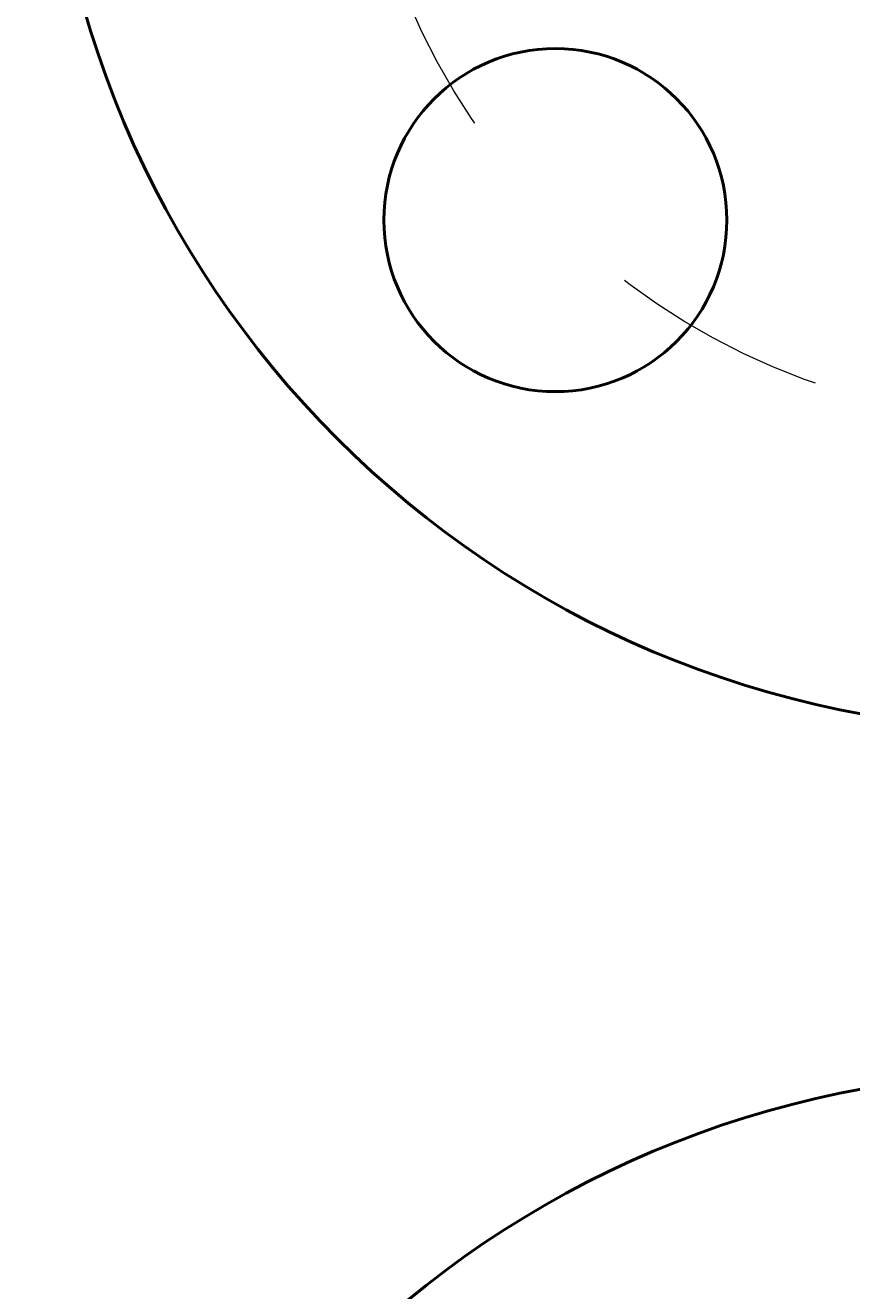
# Model space of a CAD drawing. Units: inches. Extents: x -11 to 126, y -62 to 82.
# Tile 7 of 10: x 30 to 54, y 1 to 38. Entities that reach past the tile are written whole.
import ezdxf

# ---------------------------------------------------------------- set-up
doc = ezdxf.new("R2010")
doc.units = ezdxf.units.IN
doc.header["$MEASUREMENT"] = 0
doc.linetypes.add('CENTER', pattern=[50.8, 31.75, -6.35, 6.35, -6.35])
for name, color, linetype, lineweight in [('M-CNTR', 4, 'CENTER', 18), ('M-DIMS', 2, 'Continuous', 18), ('M-OUTL', 7, 'Continuous', 50)]:
    doc.layers.add(name, color=color, linetype=linetype, lineweight=lineweight)
doc.styles.get("Standard").update_dxf_attribs({"font": 'arial.ttf'})
doc.dimstyles.get("Standard").update_dxf_attribs({"dimtxt": 0.18, "dimasz": 0.18, "dimexe": 0.18, "dimexo": 0.0625, "dimgap": 0.09, "dimtad": 0, "dimtih": 1, "dimtoh": 1, "dimdec": 4, "dimzin": 0, "dimdsep": 46, "dimtxsty": 'Standard', "dimcen": 0.09, "dimadec": 0, "dimazin": 0, "dimtfac": 1, "dimtdec": 4, "dimtofl": 0, "dimtmove": 0, "dimatfit": 3, "dimfxl": 1, "dimtolj": 1, "dimtzin": 0, "dimarcsym": 0})

# ---------------------------------------------------------------- blocks, each defined once
blk = doc.blocks.new('*U1')
blk.add_circle((0, 0), 5)
blk = doc.blocks.new('*U2')
at = {"layer": 'M-OUTL', "color": 0, "linetype": 'ByBlock', "lineweight": -2, "transparency": 16777216, "rotation": 315.0000000000001}
blk.add_blockref('*U1', (45.089, 32.212), dxfattribs=at)
blk = doc.blocks.new('*D5')
at = {"layer": 'Defpoints', "color": 0, "transparency": 16777216}
for p in [(119.232, 12.354), (-0.749, 11.479), (119.232, -57.296)]:
    blk.add_point(p, dxfattribs=at)
at = {"layer": 'M-DIMS', "color": 0, "lineweight": -2, "transparency": 16777216}
for p, q in [((119.232, 12.292), (119.232, -57.476)), ((-0.749, 11.416), (-0.749, -57.476)), ((-0.569, -57.296), (58.786, -57.296)), ((119.052, -57.296), (59.696, -57.296))]:
    blk.add_line(p, q, dxfattribs=at)
at = {"layer": 'M-DIMS', "color": 0, "transparency": 16777216}
for points in [[(-0.569, -57.266), (-0.569, -57.326), (-0.749, -57.296)], [(119.052, -57.266), (119.052, -57.326), (119.232, -57.296)]]:
    blk.add_solid(points, dxfattribs=at)
at = {"layer": 'M-DIMS', "color": 0, "transparency": 16777216, "insert": (59.241, -57.296), "char_height": 0.18, "attachment_point": 5}
blk.add_mtext('\\A1;119.98', dxfattribs=at)
blk = doc.blocks.new('*D6')
at = {"layer": 'Defpoints', "color": 0, "transparency": 16777216}
for p in [(-7.399, 75.354), (59.232, 75.354), (59.232, -50.646)]:
    blk.add_point(p, dxfattribs=at)
at = {"layer": 'M-DIMS', "color": 0, "lineweight": -2, "transparency": 16777216}
for p, q in [((59.169, 75.354), (-7.579, 75.354)), ((-7.399, 75.174), (-7.399, 12.536)), ((-7.399, -50.466), (-7.399, 12.172)), ((59.169, -50.646), (-7.579, -50.646))]:
    blk.add_line(p, q, dxfattribs=at)
at = {"layer": 'M-DIMS', "color": 0, "transparency": 16777216}
for points in [[(-7.429, 75.174), (-7.369, 75.174), (-7.399, 75.354)], [(-7.429, -50.466), (-7.369, -50.466), (-7.399, -50.646)]]:
    blk.add_solid(points, dxfattribs=at)
at = {"layer": 'M-DIMS', "color": 0, "transparency": 16777216, "insert": (-7.399, 12.354), "char_height": 0.18, "attachment_point": 5}
blk.add_mtext('\\A1;126', dxfattribs=at)
blk = doc.blocks.new('*D7')
at = {"layer": 'Defpoints', "color": 0, "transparency": 16777216}
for p in [(59.232, 82.004), (59.232, 46.354), (19.232, 12.354)]:
    blk.add_point(p, dxfattribs=at)
at = {"layer": 'M-DIMS', "color": 0, "lineweight": -2, "transparency": 16777216}
for p, q in [((19.232, 12.417), (19.232, 82.184)), ((19.412, 82.004), (39.009, 82.004)), ((59.052, 82.004), (39.454, 82.004)), ((59.232, 46.417), (59.232, 82.184))]:
    blk.add_line(p, q, dxfattribs=at)
at = {"layer": 'M-DIMS', "color": 0, "transparency": 16777216}
for points in [[(19.412, 82.034), (19.412, 81.974), (19.232, 82.004)], [(59.052, 82.034), (59.052, 81.974), (59.232, 82.004)]]:
    blk.add_solid(points, dxfattribs=at)
at = {"layer": 'M-DIMS', "color": 0, "transparency": 16777216, "insert": (39.232, 82.004), "char_height": 0.18, "attachment_point": 5}
blk.add_mtext('\\A1;40', dxfattribs=at)
blk = doc.blocks.new('*D13')
at = {"layer": 'Defpoints', "color": 0, "transparency": 16777216}
for p in [(73.731, 3.469), (44.732, -46.761)]:
    blk.add_point(p, dxfattribs=at)
at = {"layer": 'M-DIMS', "color": 0, "lineweight": -2, "transparency": 16777216}
for p, q in [((59.142, -21.646), (59.322, -21.646)), ((59.232, -21.736), (59.232, -21.556)), ((36.032, -61.83), (44.642, -46.917)), ((35.852, -61.83), (36.032, -61.83))]:
    blk.add_line(p, q, dxfattribs=at)
at = {"layer": 'M-DIMS', "color": 0, "transparency": 16777216}
blk.add_solid([(44.616, -46.902), (44.668, -46.932), (44.732, -46.761)], dxfattribs=at)
at = {"layer": 'M-DIMS', "color": 0, "transparency": 16777216, "insert": (35.345, -61.83), "char_height": 0.18, "attachment_point": 5}
blk.add_mtext('\\A1;2X ∅58', dxfattribs=at)

msp = doc.modelspace()

# ---------------------------------------------------------------- linework, layer by layer
at = {"layer": 'M-CNTR'}
msp.add_circle((59.232, 46.354), 20, dxfattribs=at)
at = {"layer": 'M-OUTL'}
for centre in [(59.232, 46.354), (59.232, -21.646)]:
    msp.add_circle(centre, 29, dxfattribs=at)

# ---------------------------------------------------------------- block references
msp.add_blockref('*U2', (0, 0), dxfattribs=at)

# ---------------------------------------------------------------- dimensions: what is measured, and where the dimension line sits
at = {"layer": 'M-DIMS'}
for base, p1, p2, override, picture, middle in [((59.232, 82.004), (19.232, 12.354), (59.232, 46.354), {"dimdec": 0, "dimlfac": 1, "dimrnd": 0, "dimzin": 0, "dimdsep": 46, "dimlunit": 2}, '*D7', (39.232, 82.004)), ((119.232, -57.296), (-0.749, 11.479), (119.232, 12.354), {"dimdec": 2, "dimlfac": 1, "dimrnd": 0, "dimzin": 0, "dimdsep": 46, "dimlunit": 2}, '*D5', (59.241, -57.296))]:
    dim = msp.add_linear_dim(base=base, p1=p1, p2=p2, dimstyle='Standard', override=override, dxfattribs=at)
    dim.commit()
    dim.dimension.update_dxf_attribs({"geometry": picture, "text_midpoint": middle})
dim = msp.add_linear_dim(base=(-7.399, 75.354), p1=(59.232, -50.646), p2=(59.232, 75.354), angle=90, dimstyle='Standard', override={"dimdec": 0, "dimlfac": 1, "dimrnd": 0, "dimzin": 0, "dimdsep": 46, "dimlunit": 2}, dxfattribs=at)
dim.commit()
dim.dimension.update_dxf_attribs({"geometry": '*D6', "text_midpoint": (-7.399, 12.354)})
dim = msp.add_diameter_dim_2p(p1=(73.731, 3.469), p2=(44.732, -46.761), text='2X <>', dimstyle='Standard', override={"dimdec": 0, "dimlfac": 1, "dimrnd": 0, "dimzin": 0, "dimdsep": 46, "dimlunit": 2}, dxfattribs=at)
dim.commit()
dim.dimension.update_dxf_attribs({"geometry": '*D13', "text_midpoint": (35.345, -61.83), "dimtype": 163})

doc.saveas('drawing.dxf')
